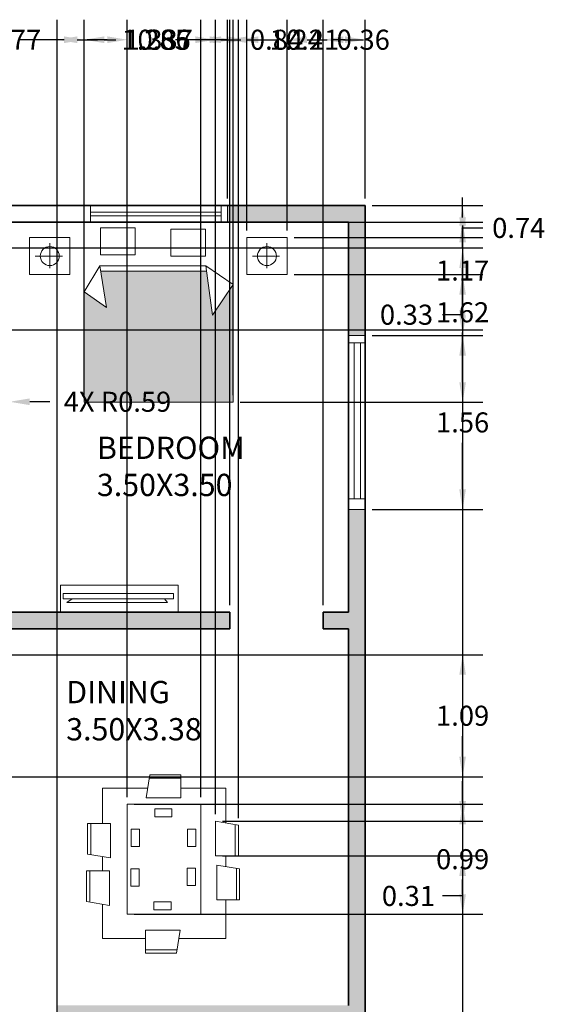
# Model space of a CAD drawing. Units: metres. Extents: x 36 to 56493, y 9 to 42849.
# Tile 5 of 5: x 56488.056 to 56492.773, y 42839.883 to 42848.722. Entities that reach past the tile are written whole.
import ezdxf

# ---------------------------------------------------------------- set-up
doc = ezdxf.new("R2010")
doc.units = ezdxf.units.M
doc.header["$MEASUREMENT"] = 0
for name, color, linetype, lineweight in [('A-ANNO-DIMS', 2, 'Continuous', 18), ('A-AREA-IDEN', 7, 'Continuous', 18), ('A-EQPM', 8, 'Continuous', 18), ('A-FURN', 8, 'Continuous', 18), ('A-FURN-PATT', 252, 'Continuous', 13), ('A-GLAZ', 4, 'Continuous', 18), ('A-WALL', 7, 'Continuous', 35)]:
    doc.layers.add(name, color=color, linetype=linetype, lineweight=lineweight)
doc.layers.add('A-WALL-PATT', color=30, linetype='Continuous', lineweight=13, true_color=0xf26722)
doc.styles.get("Standard").update_dxf_attribs({"font": 'arial.ttf'})
doc.dimstyles.get("Standard").update_dxf_attribs({"dimtxt": 0.18, "dimasz": 0.18, "dimexe": 0.18, "dimexo": 0.0625, "dimgap": 0.09, "dimtad": 0, "dimtih": 1, "dimtoh": 1, "dimdec": 0, "dimzin": 0, "dimdsep": 46, "dimtxsty": 'Standard', "dimcen": 0.09, "dimadec": 0, "dimazin": 0, "dimtfac": 1, "dimtdec": 0, "dimtofl": 0, "dimtmove": 0, "dimatfit": 3, "dimfxl": 1, "dimtolj": 1, "dimtzin": 0, "dimarcsym": 0})

# ---------------------------------------------------------------- blocks, each defined once
blk = doc.blocks.new('CHAIR-DINING')
for p, q in [((0, -0.0005), (0.0341, 0.2049)), ((0.0341, 0.2049), (0.3107, 0.2049)), ((0.3107, 0.2049), (0.3107, -0.0005)), ((0.0292, 0.1752), (0.3107, 0.1752)), ((0, -0.0005), (0.3107, -0.0005))]:
    blk.add_line(p, q)
blk = doc.blocks.new('NIGHTSTAND-COMPACT')
for p, q in [((0.1807, 0.2832), (0.1807, 0.057)), ((0.0508, 0.1663), (0.2939, 0.1663))]:
    blk.add_line(p, q)
blk.add_lwpolyline([(0, 0.3329), (0.3614, 0.3329), (0.3614, -0.0003), (0, -0.0003)], close=True)
blk.add_circle((0.1807, 0.1663), 0.0852)
blk = doc.blocks.new('*D17')
at = {"layer": 'A-ANNO-DIMS', "color": 0, "lineweight": -2, "transparency": 16777216}
for p, q in [((56491.2188, 42847.0533), (56492.2108, 42847.0533)), ((56492.0308, 42846.8733), (56492.0308, 42838.9334)), ((56492.0308, 42830.6296), (56492.0308, 42838.5695)), ((56489.3111, 42830.4496), (56492.2108, 42830.4496))]:
    blk.add_line(p, q, dxfattribs=at)
at = {"layer": 'A-ANNO-DIMS', "color": 0, "transparency": 16777216}
for points in [[(56492.0008, 42846.8733), (56492.0608, 42846.8733), (56492.0308, 42847.0533)], [(56492.0008, 42830.6296), (56492.0608, 42830.6296), (56492.0308, 42830.4496)]]:
    blk.add_solid(points, dxfattribs=at)
at = {"layer": 'Defpoints', "color": 0, "transparency": 16777216}
for p in [(56491.1563, 42847.0533), (56489.2486, 42830.4496), (56492.0308, 42830.4496)]:
    blk.add_point(p, dxfattribs=at)
at = {"layer": 'A-ANNO-DIMS', "color": 0, "transparency": 16777216, "insert": (56492.0308, 42838.7514), "char_height": 0.18, "attachment_point": 5}
blk.add_mtext('\\A1;16.604', dxfattribs=at)
blk = doc.blocks.new('*D23')
at = {"layer": 'A-ANNO-DIMS', "color": 0, "lineweight": -2, "transparency": 16777216}
for p, q in [((56489.8126, 42841.5894), (56489.8126, 42848.722)), ((56490.0179, 42841.5553), (56490.0179, 42848.722)), ((56489.6326, 42848.542), (56489.4526, 42848.542)), ((56490.1979, 42848.542), (56490.3779, 42848.542))]:
    blk.add_line(p, q, dxfattribs=at)
at = {"layer": 'A-ANNO-DIMS', "color": 0, "transparency": 16777216}
for points in [[(56489.6326, 42848.572), (56489.6326, 42848.512), (56489.8126, 42848.542)], [(56490.1979, 42848.572), (56490.1979, 42848.512), (56490.0179, 42848.542)]]:
    blk.add_solid(points, dxfattribs=at)
at = {"layer": 'Defpoints', "color": 0, "transparency": 16777216}
for p in [(56490.0179, 42848.542), (56489.8126, 42841.5269), (56490.0179, 42841.4928)]:
    blk.add_point(p, dxfattribs=at)
at = {"layer": 'A-ANNO-DIMS', "color": 0, "transparency": 16777216, "insert": (56490.6843, 42848.542), "char_height": 0.18, "attachment_point": 5}
blk.add_mtext('\\A1;0.21', dxfattribs=at)
blk = doc.blocks.new('*D24')
at = {"layer": 'A-ANNO-DIMS', "color": 0, "lineweight": -2, "transparency": 16777216}
for p, q in [((56492.0308, 42841.7069), (56492.0308, 42841.8869)), ((56489.8751, 42841.5269), (56492.2108, 42841.5269)), ((56489.8751, 42841.2162), (56492.2108, 42841.2162)), ((56492.0308, 42841.0362), (56492.0308, 42840.8562)), ((56492.0308, 42840.8562), (56491.8508, 42840.8562))]:
    blk.add_line(p, q, dxfattribs=at)
at = {"layer": 'A-ANNO-DIMS', "color": 0, "transparency": 16777216}
for points in [[(56492.0008, 42841.7069), (56492.0608, 42841.7069), (56492.0308, 42841.5269)], [(56492.0008, 42841.0362), (56492.0608, 42841.0362), (56492.0308, 42841.2162)]]:
    blk.add_solid(points, dxfattribs=at)
at = {"layer": 'Defpoints', "color": 0, "transparency": 16777216}
for p in [(56489.8126, 42841.5269), (56489.8126, 42841.2162), (56492.0308, 42841.2162)]:
    blk.add_point(p, dxfattribs=at)
at = {"layer": 'A-ANNO-DIMS', "color": 0, "transparency": 16777216, "insert": (56491.5443, 42840.8562), "char_height": 0.18, "attachment_point": 5}
blk.add_mtext('\\A1;0.31', dxfattribs=at)
blk = doc.blocks.new('*D27')
at = {"layer": 'A-ANNO-DIMS', "color": 0, "lineweight": -2, "transparency": 16777216}
for p, q in [((56490.094, 42846.8294), (56490.094, 42848.722)), ((56490.4554, 42846.8294), (56490.4554, 42848.722)), ((56489.914, 42848.542), (56489.734, 42848.542)), ((56490.6354, 42848.542), (56490.8154, 42848.542))]:
    blk.add_line(p, q, dxfattribs=at)
at = {"layer": 'A-ANNO-DIMS', "color": 0, "transparency": 16777216}
for points in [[(56489.914, 42848.572), (56489.914, 42848.512), (56490.094, 42848.542)], [(56490.6354, 42848.572), (56490.6354, 42848.512), (56490.4554, 42848.542)]]:
    blk.add_solid(points, dxfattribs=at)
at = {"layer": 'Defpoints', "color": 0, "transparency": 16777216}
for p in [(56490.4554, 42848.542), (56490.094, 42846.7669), (56490.4554, 42846.7669)]:
    blk.add_point(p, dxfattribs=at)
at = {"layer": 'A-ANNO-DIMS', "color": 0, "transparency": 16777216, "insert": (56491.1391, 42848.542), "char_height": 0.18, "attachment_point": 5}
blk.add_mtext('\\A1;0.36', dxfattribs=at)
blk = doc.blocks.new('*D28')
at = {"layer": 'A-ANNO-DIMS', "color": 0, "lineweight": -2, "transparency": 16777216}
for p, q in [((56492.030752, 42846.94694), (56492.030752, 42847.12694)), ((56490.517921, 42846.76694), (56492.210752, 42846.76694)), ((56490.517921, 42846.433723), (56492.210752, 42846.433723)), ((56492.030752, 42846.253723), (56492.030752, 42846.073723)), ((56492.030752, 42846.073723), (56491.850752, 42846.073723))]:
    blk.add_line(p, q, dxfattribs=at)
at = {"layer": 'A-ANNO-DIMS', "color": 0, "transparency": 16777216}
for points in [[(56492.000752, 42846.94694), (56492.060752, 42846.94694), (56492.030752, 42846.76694)], [(56492.000752, 42846.253723), (56492.060752, 42846.253723), (56492.030752, 42846.433723)]]:
    blk.add_solid(points, dxfattribs=at)
at = {"layer": 'Defpoints', "color": 0, "transparency": 16777216}
for p in [(56490.455421, 42846.76694), (56490.455421, 42846.433723), (56492.030752, 42846.433723)]:
    blk.add_point(p, dxfattribs=at)
at = {"layer": 'A-ANNO-DIMS', "color": 0, "transparency": 16777216, "insert": (56491.526973, 42846.073723), "char_height": 0.18, "attachment_point": 5}
blk.add_mtext('\\A1;0.33', dxfattribs=at)
blk = doc.blocks.new('*D45')
at = {"layer": 'A-ANNO-DIMS', "color": 0, "lineweight": -2, "transparency": 16777216}
for p, q in [((56486.6826, 42847.1158), (56486.6826, 42848.722)), ((56488.6347, 42847.1158), (56488.6347, 42848.722)), ((56486.8626, 42848.542), (56487.2744, 42848.542)), ((56488.4547, 42848.542), (56488.043, 42848.542))]:
    blk.add_line(p, q, dxfattribs=at)
at = {"layer": 'A-ANNO-DIMS', "color": 0, "transparency": 16777216}
for points in [[(56486.8626, 42848.572), (56486.8626, 42848.512), (56486.6826, 42848.542)], [(56488.4547, 42848.572), (56488.4547, 42848.512), (56488.6347, 42848.542)]]:
    blk.add_solid(points, dxfattribs=at)
at = {"layer": 'Defpoints', "color": 0, "transparency": 16777216}
for p in [(56488.6347, 42848.542), (56486.6826, 42847.0533), (56488.6347, 42847.0533)]:
    blk.add_point(p, dxfattribs=at)
at = {"layer": 'A-ANNO-DIMS', "color": 0, "transparency": 16777216, "insert": (56487.6587, 42848.542), "char_height": 0.18, "attachment_point": 5}
blk.add_mtext('\\A1;1.952', dxfattribs=at)
blk = doc.blocks.new('*D46')
at = {"layer": 'A-ANNO-DIMS', "color": 0, "lineweight": -2, "transparency": 16777216}
for p, q in [((56488.6347, 42847.1158), (56488.6347, 42848.722)), ((56489.9198, 42847.1158), (56489.9198, 42848.722)), ((56488.4547, 42848.542), (56488.2747, 42848.542)), ((56490.0998, 42848.542), (56490.2798, 42848.542))]:
    blk.add_line(p, q, dxfattribs=at)
at = {"layer": 'A-ANNO-DIMS', "color": 0, "transparency": 16777216}
for points in [[(56488.4547, 42848.572), (56488.4547, 42848.512), (56488.6347, 42848.542)], [(56490.0998, 42848.572), (56490.0998, 42848.512), (56489.9198, 42848.542)]]:
    blk.add_solid(points, dxfattribs=at)
at = {"layer": 'Defpoints', "color": 0, "transparency": 16777216}
for p in [(56489.9198, 42848.542), (56488.6347, 42847.0533), (56489.9198, 42847.0533)]:
    blk.add_point(p, dxfattribs=at)
at = {"layer": 'A-ANNO-DIMS', "color": 0, "transparency": 16777216, "insert": (56489.2773, 42848.542), "char_height": 0.18, "attachment_point": 5}
blk.add_mtext('\\A1;1.285', dxfattribs=at)
blk = doc.blocks.new('*D47')
at = {"layer": 'A-ANNO-DIMS', "color": 0, "lineweight": -2, "transparency": 16777216}
for p, q in [((56489.9198, 42847.1158), (56489.9198, 42848.722)), ((56491.1563, 42847.1158), (56491.1563, 42848.722)), ((56490.0998, 42848.542), (56490.2231, 42848.542)), ((56490.9763, 42848.542), (56490.853, 42848.542))]:
    blk.add_line(p, q, dxfattribs=at)
at = {"layer": 'A-ANNO-DIMS', "color": 0, "transparency": 16777216}
for points in [[(56490.0998, 42848.572), (56490.0998, 42848.512), (56489.9198, 42848.542)], [(56490.9763, 42848.572), (56490.9763, 42848.512), (56491.1563, 42848.542)]]:
    blk.add_solid(points, dxfattribs=at)
at = {"layer": 'Defpoints', "color": 0, "transparency": 16777216}
for p in [(56491.1563, 42848.542), (56489.9198, 42847.0533), (56491.1563, 42847.0533)]:
    blk.add_point(p, dxfattribs=at)
at = {"layer": 'A-ANNO-DIMS', "color": 0, "transparency": 16777216, "insert": (56490.538, 42848.542), "char_height": 0.18, "attachment_point": 5}
blk.add_mtext('\\A1;1.24', dxfattribs=at)
blk = doc.blocks.new('*D54')
at = {"layer": 'A-ANNO-DIMS', "color": 0, "lineweight": -2, "transparency": 16777216}
for p, q in [((56491.2188, 42847.0533), (56492.2108, 42847.0533)), ((56492.0308, 42846.8733), (56492.0308, 42846.6505)), ((56492.0308, 42846.067), (56492.0308, 42846.2898)), ((56491.2188, 42845.887), (56492.2108, 42845.887))]:
    blk.add_line(p, q, dxfattribs=at)
at = {"layer": 'A-ANNO-DIMS', "color": 0, "transparency": 16777216}
for points in [[(56492.0008, 42846.8733), (56492.0608, 42846.8733), (56492.0308, 42847.0533)], [(56492.0008, 42846.067), (56492.0608, 42846.067), (56492.0308, 42845.887)]]:
    blk.add_solid(points, dxfattribs=at)
at = {"layer": 'Defpoints', "color": 0, "transparency": 16777216}
for p in [(56491.1563, 42847.0533), (56491.1563, 42845.887), (56492.0308, 42845.887)]:
    blk.add_point(p, dxfattribs=at)
at = {"layer": 'A-ANNO-DIMS', "color": 0, "transparency": 16777216, "insert": (56492.0308, 42846.4701), "char_height": 0.18, "attachment_point": 5}
blk.add_mtext('\\A1;1.17', dxfattribs=at)
blk = doc.blocks.new('*D55')
at = {"layer": 'A-ANNO-DIMS', "color": 0, "lineweight": -2, "transparency": 16777216}
for p, q in [((56491.2188, 42845.887), (56492.2108, 42845.887)), ((56492.0308, 42845.707), (56492.0308, 42845.2886)), ((56492.0308, 42844.5064), (56492.0308, 42844.9248)), ((56491.2188, 42844.3264), (56492.2108, 42844.3264))]:
    blk.add_line(p, q, dxfattribs=at)
at = {"layer": 'A-ANNO-DIMS', "color": 0, "transparency": 16777216}
for points in [[(56492.0008, 42845.707), (56492.0608, 42845.707), (56492.0308, 42845.887)], [(56492.0008, 42844.5064), (56492.0608, 42844.5064), (56492.0308, 42844.3264)]]:
    blk.add_solid(points, dxfattribs=at)
at = {"layer": 'Defpoints', "color": 0, "transparency": 16777216}
for p in [(56491.1563, 42845.887), (56491.1563, 42844.3264), (56492.0308, 42844.3264)]:
    blk.add_point(p, dxfattribs=at)
at = {"layer": 'A-ANNO-DIMS', "color": 0, "transparency": 16777216, "insert": (56492.0308, 42845.1067), "char_height": 0.18, "attachment_point": 5}
blk.add_mtext('\\A1;1.56', dxfattribs=at)
blk = doc.blocks.new('*D58')
at = {"layer": 'A-ANNO-DIMS', "color": 0, "lineweight": -2, "transparency": 16777216}
for p, q in [((56488.6347, 42845.3504), (56488.6347, 42848.722)), ((56489.9717, 42845.3504), (56489.9717, 42848.722)), ((56488.8147, 42848.542), (56488.918, 42848.542)), ((56489.7917, 42848.542), (56489.6885, 42848.542))]:
    blk.add_line(p, q, dxfattribs=at)
at = {"layer": 'A-ANNO-DIMS', "color": 0, "transparency": 16777216}
for points in [[(56488.8147, 42848.572), (56488.8147, 42848.512), (56488.6347, 42848.542)], [(56489.7917, 42848.572), (56489.7917, 42848.512), (56489.9717, 42848.542)]]:
    blk.add_solid(points, dxfattribs=at)
at = {"layer": 'Defpoints', "color": 0, "transparency": 16777216}
for p in [(56489.9717, 42848.542), (56488.6347, 42845.2879), (56489.9717, 42845.2879)]:
    blk.add_point(p, dxfattribs=at)
at = {"layer": 'A-ANNO-DIMS', "color": 0, "transparency": 16777216, "insert": (56489.3032, 42848.542), "char_height": 0.18, "attachment_point": 5}
blk.add_mtext('\\A1;1.337', dxfattribs=at)
blk = doc.blocks.new('*D59')
at = {"layer": 'A-ANNO-DIMS', "color": 0, "lineweight": -2, "transparency": 16777216}
for p, q in [((56490.0342, 42846.9033), (56492.2108, 42846.9033)), ((56492.0308, 42846.7233), (56492.0308, 42846.2775)), ((56492.0308, 42845.4679), (56492.0308, 42845.9137)), ((56490.0342, 42845.2879), (56492.2108, 42845.2879))]:
    blk.add_line(p, q, dxfattribs=at)
at = {"layer": 'A-ANNO-DIMS', "color": 0, "transparency": 16777216}
for points in [[(56492.0008, 42846.7233), (56492.0608, 42846.7233), (56492.0308, 42846.9033)], [(56492.0008, 42845.4679), (56492.0608, 42845.4679), (56492.0308, 42845.2879)]]:
    blk.add_solid(points, dxfattribs=at)
at = {"layer": 'Defpoints', "color": 0, "transparency": 16777216}
for p in [(56489.9717, 42846.9033), (56492.0308, 42846.9033), (56489.9717, 42845.2879)]:
    blk.add_point(p, dxfattribs=at)
at = {"layer": 'A-ANNO-DIMS', "color": 0, "transparency": 16777216, "insert": (56492.0308, 42846.0956), "char_height": 0.18, "attachment_point": 5}
blk.add_mtext('\\A1;1.62', dxfattribs=at)
blk = doc.blocks.new('*D60')
at = {"layer": 'A-ANNO-DIMS', "color": 0, "lineweight": -2, "transparency": 16777216}
for p, q in [((56489.021472, 42841.742527), (56489.021472, 42848.721953)), ((56489.681318, 42841.742527), (56489.681318, 42848.721953)), ((56488.841472, 42848.541953), (56488.661472, 42848.541953)), ((56489.861318, 42848.541953), (56490.041318, 42848.541953))]:
    blk.add_line(p, q, dxfattribs=at)
at = {"layer": 'A-ANNO-DIMS', "color": 0, "transparency": 16777216}
for points in [[(56488.841472, 42848.571953), (56488.841472, 42848.511953), (56489.021472, 42848.541953)], [(56489.861318, 42848.571953), (56489.861318, 42848.511953), (56489.681318, 42848.541953)]]:
    blk.add_solid(points, dxfattribs=at)
at = {"layer": 'Defpoints', "color": 0, "transparency": 16777216}
for p in [(56489.681318, 42848.541953), (56489.021472, 42841.680027), (56489.681318, 42841.680027)]:
    blk.add_point(p, dxfattribs=at)
at = {"layer": 'A-ANNO-DIMS', "color": 0, "transparency": 16777216, "insert": (56489.351395, 42848.541953), "char_height": 0.18, "attachment_point": 5}
blk.add_mtext('\\A1;0.66', dxfattribs=at)
blk = doc.blocks.new('*D61')
at = {"layer": 'A-ANNO-DIMS', "color": 0, "lineweight": -2, "transparency": 16777216}
for p, q in [((56489.084, 42841.68), (56492.2108, 42841.68)), ((56492.0308, 42841.5), (56492.0308, 42841.3677)), ((56492.0308, 42840.8715), (56492.0308, 42841.0039)), ((56489.084, 42840.6915), (56492.2108, 42840.6915))]:
    blk.add_line(p, q, dxfattribs=at)
at = {"layer": 'A-ANNO-DIMS', "color": 0, "transparency": 16777216}
for points in [[(56492.0008, 42841.5), (56492.0608, 42841.5), (56492.0308, 42841.68)], [(56492.0008, 42840.8715), (56492.0608, 42840.8715), (56492.0308, 42840.6915)]]:
    blk.add_solid(points, dxfattribs=at)
at = {"layer": 'Defpoints', "color": 0, "transparency": 16777216}
for p in [(56489.0215, 42841.68), (56489.0215, 42840.6915), (56492.0308, 42840.6915)]:
    blk.add_point(p, dxfattribs=at)
at = {"layer": 'A-ANNO-DIMS', "color": 0, "transparency": 16777216, "insert": (56492.0308, 42841.1858), "char_height": 0.18, "attachment_point": 5}
blk.add_mtext('\\A1;0.99', dxfattribs=at)
blk = doc.blocks.new('*D63')
at = {"layer": 'A-ANNO-DIMS', "color": 0, "lineweight": -2, "transparency": 16777216}
for p, q in [((56492.0308, 42846.6728), (56492.0308, 42846.8528)), ((56492.0308, 42846.8528), (56492.2108, 42846.8528)), ((56487.4188, 42846.6728), (56492.2108, 42846.6728)), ((56492.0308, 42846.1166), (56492.0308, 42846.4928)), ((56487.4188, 42845.9366), (56492.2108, 42845.9366))]:
    blk.add_line(p, q, dxfattribs=at)
at = {"layer": 'A-ANNO-DIMS', "color": 0, "transparency": 16777216}
for points in [[(56492.0008, 42846.4928), (56492.0608, 42846.4928), (56492.0308, 42846.6728)], [(56492.0008, 42846.1166), (56492.0608, 42846.1166), (56492.0308, 42845.9366)]]:
    blk.add_solid(points, dxfattribs=at)
at = {"layer": 'Defpoints', "color": 0, "transparency": 16777216}
for p in [(56487.3563, 42846.6728), (56492.0308, 42846.6728), (56487.3563, 42845.9366)]:
    blk.add_point(p, dxfattribs=at)
at = {"layer": 'A-ANNO-DIMS', "color": 0, "transparency": 16777216, "insert": (56492.5342, 42846.8528), "char_height": 0.18, "attachment_point": 5}
blk.add_mtext('\\A1;0.74', dxfattribs=at)
blk = doc.blocks.new('*D64')
at = {"layer": 'A-ANNO-DIMS', "color": 0, "lineweight": -2, "transparency": 16777216}
for p, q in [((56487.4188, 42843.021), (56492.2108, 42843.021)), ((56492.0308, 42842.841), (56492.0308, 42842.6556)), ((56492.0308, 42842.1064), (56492.0308, 42842.2918)), ((56487.4188, 42841.9264), (56492.2108, 42841.9264))]:
    blk.add_line(p, q, dxfattribs=at)
at = {"layer": 'A-ANNO-DIMS', "color": 0, "transparency": 16777216}
for points in [[(56492.0008, 42842.841), (56492.0608, 42842.841), (56492.0308, 42843.021)], [(56492.0008, 42842.1064), (56492.0608, 42842.1064), (56492.0308, 42841.9264)]]:
    blk.add_solid(points, dxfattribs=at)
at = {"layer": 'Defpoints', "color": 0, "transparency": 16777216}
for p in [(56487.3563, 42843.021), (56487.3563, 42841.9264), (56492.0308, 42841.9264)]:
    blk.add_point(p, dxfattribs=at)
at = {"layer": 'A-ANNO-DIMS', "color": 0, "transparency": 16777216, "insert": (56492.0308, 42842.4737), "char_height": 0.18, "attachment_point": 5}
blk.add_mtext('\\A1;1.09', dxfattribs=at)
blk = doc.blocks.new('*D65')
at = {"layer": 'A-ANNO-DIMS', "color": 0, "lineweight": -2, "transparency": 16777216}
for p, q in [((56489.940126, 42843.465791), (56489.940126, 42848.721953)), ((56490.780472, 42843.465791), (56490.780472, 42848.721953)), ((56489.760126, 42848.541953), (56489.580126, 42848.541953)), ((56490.960472, 42848.541953), (56491.140472, 42848.541953))]:
    blk.add_line(p, q, dxfattribs=at)
at = {"layer": 'A-ANNO-DIMS', "color": 0, "transparency": 16777216}
for points in [[(56489.760126, 42848.571953), (56489.760126, 42848.511953), (56489.940126, 42848.541953)], [(56490.960472, 42848.571953), (56490.960472, 42848.511953), (56490.780472, 42848.541953)]]:
    blk.add_solid(points, dxfattribs=at)
at = {"layer": 'Defpoints', "color": 0, "transparency": 16777216}
for p in [(56490.780472, 42848.541953), (56489.940126, 42843.403291), (56490.780472, 42843.403291)]:
    blk.add_point(p, dxfattribs=at)
at = {"layer": 'A-ANNO-DIMS', "color": 0, "transparency": 16777216, "insert": (56490.360299, 42848.541953), "char_height": 0.18, "attachment_point": 5}
blk.add_mtext('\\A1;0.84', dxfattribs=at)
blk = doc.blocks.new('*D67')
at = {"layer": 'A-ANNO-DIMS', "color": 0, "lineweight": -2, "transparency": 16777216}
for p, q in [((56487.626252, 42839.785791), (56487.626252, 42848.721953)), ((56488.392626, 42839.785791), (56488.392626, 42848.721953)), ((56487.446252, 42848.541953), (56487.266252, 42848.541953)), ((56488.572626, 42848.541953), (56488.752626, 42848.541953))]:
    blk.add_line(p, q, dxfattribs=at)
at = {"layer": 'A-ANNO-DIMS', "color": 0, "transparency": 16777216}
for points in [[(56487.446252, 42848.571953), (56487.446252, 42848.511953), (56487.626252, 42848.541953)], [(56488.572626, 42848.571953), (56488.572626, 42848.511953), (56488.392626, 42848.541953)]]:
    blk.add_solid(points, dxfattribs=at)
at = {"layer": 'Defpoints', "color": 0, "transparency": 16777216}
for p in [(56488.392626, 42848.541953), (56487.626252, 42839.723291), (56488.392626, 42839.723291)]:
    blk.add_point(p, dxfattribs=at)
at = {"layer": 'A-ANNO-DIMS', "color": 0, "transparency": 16777216, "insert": (56488.009439, 42848.541953), "char_height": 0.18, "attachment_point": 5}
blk.add_mtext('\\A1;0.77', dxfattribs=at)
blk = doc.blocks.new('*D71')
at = {"layer": 'A-ANNO-DIMS', "color": 0, "lineweight": -2, "transparency": 16777216}
for p, q in [((56487.3732, 42845.2016), (56487.3732, 42845.3816)), ((56487.2832, 42845.2916), (56487.4632, 42845.2916)), ((56488.3266, 42845.2922), (56488.1466, 42845.2921))]:
    blk.add_line(p, q, dxfattribs=at)
at = {"layer": 'A-ANNO-DIMS', "color": 0, "transparency": 16777216}
blk.add_solid([(56488.1466, 42845.3221), (56488.1466, 42845.2621), (56487.9666, 42845.292)], dxfattribs=at)
at = {"layer": 'Defpoints', "color": 0, "transparency": 16777216}
for p in [(56487.3732, 42845.2916), (56487.9666, 42845.292)]:
    blk.add_point(p, dxfattribs=at)
at = {"layer": 'A-ANNO-DIMS', "color": 0, "transparency": 16777216, "insert": (56488.9337, 42845.2922), "char_height": 0.18, "attachment_point": 5}
blk.add_mtext('\\A1;4X R0.59', dxfattribs=at)

msp = doc.modelspace()

# ---------------------------------------------------------------- hatches: boundary and pattern name
at = {"layer": 'A-FURN-PATT'}
h = msp.add_hatch(color=256, dxfattribs=at)
h.dxf.hatch_style = 1
h.paths.add_polyline_path([(56489.9717, 42846.3436), (56489.785, 42846.0689), (56489.7313, 42846.464), (56488.7831, 42846.4638), (56488.8356, 42846.1393), (56488.6347, 42846.2795), (56488.6347, 42845.2879), (56489.9717, 42845.2879)])
at = {"layer": 'A-WALL-PATT'}
h = msp.add_hatch(color=256, dxfattribs=at)
h.dxf.hatch_style = 1
edge = h.paths.add_edge_path()
edge.add_line((56483.5429, 42845.6533), (56483.4063, 42845.6533))
edge.add_line((56483.4063, 42845.6533), (56483.4063, 42846.9033))
edge.add_line((56483.4063, 42846.9033), (56483.63, 42846.9033))
edge.add_ellipse((56483.6664, 42846.7323), major_axis=(0.2141, -0.003), ratio=0.809245, start_angle=94.07135, end_angle=102.818, ccw=False)
edge.add_line((56483.6565, 42846.9062), (56483.6565, 42846.9056))
edge.add_line((56483.6565, 42846.9056), (56483.6615, 42846.9056))
edge.add_ellipse((56483.6664, 42846.7323), major_axis=(0.2141, -0.003), ratio=0.809245, start_angle=90, end_angle=92.42655, ccw=False)
edge.add_line((56483.6812, 42846.9058), (56483.6812, 42846.9052))
edge.add_ellipse((56483.6664, 42846.7323), major_axis=(0.2141, -0.003), ratio=0.809245, start_angle=79.57494, end_angle=85.92601, ccw=False)
edge.add_line((56483.7048, 42846.9033), (56484.1418, 42846.9033))
edge.add_line((56484.1418, 42846.9033), (56484.1418, 42847.0533))
edge.add_line((56484.1418, 42847.0533), (56483.2563, 42847.0533))
edge.add_line((56483.2563, 42847.0533), (56483.2563, 42844.1391))
edge.add_line((56483.2563, 42844.1391), (56483.4063, 42844.1391))
edge.add_line((56483.4063, 42844.1391), (56483.4063, 42844.2368))
edge.add_line((56483.4063, 42844.2368), (56483.4063, 42845.5033))
edge.add_line((56483.4063, 42845.5033), (56483.5429, 42845.5033))
edge.add_line((56483.5429, 42845.5033), (56483.5429, 42845.6533))
edge = h.paths.add_edge_path(flags=0)
edge.add_line((56488.6347, 42847.0533), (56486.6826, 42847.0533))
edge.add_line((56486.6826, 42847.0533), (56486.6826, 42846.9033))
edge.add_line((56486.6826, 42846.9033), (56486.9892, 42846.9033))
edge.add_ellipse((56487.0257, 42846.7323), major_axis=(0.2141, -0.003), ratio=0.809245, start_angle=94.07135, end_angle=102.818, ccw=False)
edge.add_line((56487.0157, 42846.9062), (56487.0157, 42846.9056))
edge.add_line((56487.0157, 42846.9056), (56487.0207, 42846.9056))
edge.add_ellipse((56487.0257, 42846.7323), major_axis=(0.2141, -0.003), ratio=0.809245, start_angle=90, end_angle=92.42655, ccw=False)
edge.add_line((56487.0404, 42846.9058), (56487.0404, 42846.9052))
edge.add_ellipse((56487.0257, 42846.7323), major_axis=(0.2141, -0.003), ratio=0.809245, start_angle=79.57494, end_angle=85.92601, ccw=False)
edge.add_line((56487.064, 42846.9033), (56487.3563, 42846.9033))
edge.add_line((56487.3563, 42846.9033), (56487.3563, 42846.6728))
edge.add_line((56487.3563, 42846.6728), (56487.5063, 42846.6728))
edge.add_line((56487.5063, 42846.6728), (56487.5063, 42846.9033))
edge.add_line((56487.5063, 42846.9033), (56488.6347, 42846.9033))
edge.add_line((56488.6347, 42846.9033), (56488.6347, 42847.0533))
h.paths.add_polyline_path([(56486.2245, 42847.0533), (56484.665, 42847.0533), (56484.665, 42846.9033), (56485.4063, 42846.9033), (56485.4063, 42845.6533), (56484.2087, 42845.6533), (56484.2087, 42845.5033), (56487.3563, 42845.5033), (56487.3563, 42844.954), (56487.3563, 42843.021), (56487.5063, 42843.021), (56487.5063, 42843.2533), (56489.9401, 42843.2533), (56489.9401, 42843.4033), (56487.5063, 42843.4033), (56487.5063, 42845.6238), (56487.5063, 42845.6533), (56487.5063, 42845.9366), (56487.3563, 42845.9366), (56487.3563, 42845.6533), (56485.5563, 42845.6533), (56485.5563, 42846.9033), (56486.2245, 42846.9033)])
h.paths.add_polyline_path([(56491.1563, 42847.0533), (56489.9198, 42847.0533), (56489.9198, 42846.9033), (56489.9717, 42846.9033), (56491.0063, 42846.9033), (56491.0063, 42845.887), (56491.1563, 42845.887)])
h.paths.add_polyline_path([(56491.1563, 42844.3264), (56491.0063, 42844.3264), (56491.0063, 42843.4033), (56490.7805, 42843.4033), (56490.7805, 42843.2533), (56491.0063, 42843.2533), (56491.0063, 42839.8733), (56488.3926, 42839.8733), (56488.3926, 42839.7233), (56491.0063, 42839.7233), (56491.0063, 42836.1233), (56487.6263, 42836.1233), (56487.6263, 42839.0009), (56487.4763, 42839.0009), (56487.4763, 42836.1233), (56486.4863, 42836.1233), (56486.4863, 42835.9733), (56487.4763, 42835.9733), (56487.8849, 42835.9733), (56487.8849, 42832.9233), (56487.8913, 42832.9233), (56488.0349, 42832.9233), (56488.0349, 42833.0733), (56488.0349, 42835.9733), (56491.0063, 42835.9733), (56491.0063, 42833.0733), (56491.0063, 42832.9233), (56491.1563, 42832.9233), (56491.1563, 42835.9733)])
h.paths.add_polyline_path([(56483.4063, 42842.8378), (56483.2563, 42842.8378), (56483.2563, 42841.5433), (56483.2563, 42840.8898), (56483.4063, 42840.8898), (56483.4063, 42841.3933), (56485.0063, 42841.3933), (56485.0063, 42841.2426), (56485.1563, 42841.2426), (56485.1563, 42841.3933), (56487.3563, 42841.3933), (56487.5063, 42841.3933), (56487.5063, 42841.9264), (56487.3563, 42841.9264), (56487.3563, 42841.5433), (56483.4063, 42841.5433)])
h.paths.add_polyline_path([(56485.1563, 42840.351), (56485.0063, 42840.351), (56485.0063, 42839.8933), (56483.4063, 42839.8933), (56483.4063, 42840.3779), (56483.2563, 42840.3779), (56483.2563, 42839.8933), (56483.2563, 42838.6997), (56483.4063, 42838.6997), (56483.4063, 42839.7433), (56485.1563, 42839.7433)])
h.paths.add_polyline_path([(56483.4063, 42836.7612), (56483.2563, 42836.7612), (56483.2563, 42835.6733), (56483.2563, 42834.2533), (56483.2563, 42832.9233), (56485.9871, 42832.9233), (56485.9871, 42833.0733), (56483.4063, 42833.0733), (56483.4063, 42834.2533), (56483.4063, 42835.5233), (56485.4763, 42835.5233), (56485.9871, 42835.5233), (56485.9871, 42835.6733), (56485.6263, 42835.6733), (56483.4063, 42835.6733)])

# ---------------------------------------------------------------- linework, layer by layer
at = {"layer": 'A-EQPM'}
for p, q in [((56488.5276, 42843.5246), (56488.4796, 42843.4911)), ((56488.4796, 42843.4911), (56489.3827, 42843.4911)), ((56489.3827, 42843.4911), (56489.3543, 42843.5246))]:
    msp.add_line(p, q, dxfattribs=at)
for points in [[(56488.4205, 42843.4033), (56489.4788, 42843.4033), (56489.4788, 42843.6458), (56488.4205, 42843.6458)], [(56488.4465, 42843.5711), (56489.4359, 42843.5711), (56489.4359, 42843.5246), (56488.4465, 42843.5246)]]:
    msp.add_lwpolyline(points, close=True, dxfattribs=at)
at = {"layer": 'A-FURN'}
for p, q in [((56488.7754, 42846.5115), (56488.6347, 42846.2795)), ((56488.7754, 42846.5115), (56489.7249, 42846.5115)), ((56488.8356, 42846.1393), (56488.7754, 42846.5115)), ((56489.7249, 42846.5115), (56489.9717, 42846.3436)), ((56489.785, 42846.0689), (56489.7249, 42846.5115)), ((56488.7831, 42846.4638), (56489.7313, 42846.464)), ((56489.9717, 42846.3436), (56489.785, 42846.0689)), ((56488.6347, 42846.2795), (56488.8356, 42846.1393))]:
    msp.add_line(p, q, dxfattribs=at)
for points in [[(56488.6347, 42846.9033), (56489.9717, 42846.9033), (56489.9717, 42845.2879), (56488.6347, 42845.2879)], [(56488.7796, 42846.8538), (56489.0914, 42846.8538), (56489.0914, 42846.6116), (56488.7796, 42846.6116)], [(56489.4128, 42846.8407), (56489.7246, 42846.8407), (56489.7246, 42846.5985), (56489.4128, 42846.5985)], [(56489.0215, 42841.68), (56489.6813, 42841.68), (56489.6813, 42840.6915), (56489.0215, 42840.6915)], [(56489.2673, 42841.6387), (56489.4225, 42841.6387), (56489.4225, 42841.5648), (56489.2673, 42841.5648)], [(56489.1311, 42841.454), (56489.1311, 42841.2988), (56489.0573, 42841.2988), (56489.0573, 42841.454)], [(56489.6363, 42841.4564), (56489.6363, 42841.3011), (56489.5624, 42841.3011), (56489.5624, 42841.4564)], [(56489.1264, 42841.098), (56489.1264, 42840.9427), (56489.0525, 42840.9427), (56489.0525, 42841.098)], [(56489.6339, 42841.1051), (56489.6339, 42840.9498), (56489.5601, 42840.9498), (56489.5601, 42841.1051)], [(56489.2608, 42840.8042), (56489.4161, 42840.8042), (56489.4161, 42840.7304), (56489.2608, 42840.7304)]]:
    msp.add_lwpolyline(points, close=True, dxfattribs=at)
for points in [[(56488.7998, 42841.5077), (56488.7998, 42841.8244), (56489.2054, 42841.8244)], [(56489.5017, 42841.8244), (56489.9055, 42841.8244), (56489.9055, 42841.5114)], [(56488.7998, 42841.0822), (56488.7998, 42841.2087)], [(56489.9055, 42841.2162), (56489.9055, 42841.1186)], [(56489.9055, 42840.8214), (56489.9055, 42840.4726), (56489.4836, 42840.4726)], [(56489.1855, 42840.4726), (56488.7998, 42840.4726), (56488.7998, 42840.7818)]]:
    msp.add_lwpolyline(points, dxfattribs=at)
at = {"layer": 'A-GLAZ'}
for p, q in [((56488.6347, 42847.0533), (56488.6347, 42846.9033)), ((56488.6908, 42847.0533), (56488.6908, 42846.9033)), ((56489.8629, 42847.0533), (56489.8629, 42846.9033)), ((56489.9198, 42847.0533), (56489.9198, 42846.9033)), ((56488.6908, 42846.994), (56489.8629, 42846.994)), ((56488.6908, 42846.961), (56489.8629, 42846.961)), ((56491.0063, 42845.887), (56491.1563, 42845.887)), ((56491.0063, 42845.8203), (56491.1563, 42845.8203)), ((56491.0565, 42845.8203), (56491.0565, 42844.4215)), ((56491.1143, 42845.8203), (56491.1143, 42844.4215)), ((56491.0063, 42844.4215), (56491.1563, 42844.4215)), ((56491.0063, 42844.3264), (56491.1563, 42844.3264))]:
    msp.add_line(p, q, dxfattribs=at)
at = {"layer": 'A-WALL'}
for p, q in [((56483.2563, 42847.0533), (56491.1563, 42847.0533)), ((56491.1563, 42847.0533), (56491.1563, 42843.4033)), ((56491.1563, 42847.0533), (56491.1563, 42832.9233)), ((56487.5063, 42846.9033), (56491.0063, 42846.9033)), ((56491.0063, 42846.9033), (56491.0063, 42843.4033)), ((56489.9401, 42843.4033), (56487.5063, 42843.4033)), ((56489.9401, 42843.4033), (56489.9401, 42843.2533)), ((56491.0063, 42843.4033), (56490.7805, 42843.4033)), ((56490.7805, 42843.4033), (56490.7805, 42843.2533)), ((56489.9401, 42843.2533), (56487.5063, 42843.2533)), ((56491.0063, 42843.2533), (56490.7805, 42843.2533)), ((56491.0063, 42843.2533), (56491.0063, 42839.8733))]:
    msp.add_line(p, q, dxfattribs=at)

# ---------------------------------------------------------------- block references
at = {"layer": 'A-FURN'}
for name, p in [('NIGHTSTAND-COMPACT', (56488.1449, 42846.434)), ('NIGHTSTAND-COMPACT', (56490.094, 42846.434)), ('CHAIR-DINING', (56489.191, 42841.738))]:
    msp.add_blockref(name, p, dxfattribs=at)
for p, rotation in [((56489.8131, 42841.5269), 270.0000000102918), ((56488.8696, 42841.197), 90), ((56489.8249, 42841.1321), 270.0000000057421), ((56488.861, 42840.7716), 90.0000000004862), ((56489.4962, 42840.5478), 180)]:
    msp.add_blockref('CHAIR-DINING', p, dxfattribs=dict(at, rotation=rotation))

# ---------------------------------------------------------------- texts
at = {"layer": 'A-AREA-IDEN', "char_height": 0.2, "attachment_point": 1}
for s, insert in [('BEDROOM\\P3.50X3.50', (56488.7487, 42844.9789)), ('DINING\\P3.50X3.38', (56488.473, 42842.786))]:
    msp.add_mtext_dynamic_manual_height_columns(s, width=0.817901, gutter_width=1, heights=[0], dxfattribs=dict(at, insert=insert))

# ---------------------------------------------------------------- dimensions: what is measured, and where the dimension line sits
at = {"layer": 'A-ANNO-DIMS'}
for base, p1, p2, override, picture, middle in [((56488.6347, 42848.542), (56486.6826, 42847.0533), (56488.6347, 42847.0533), {"dimdec": 3, "dimlfac": 1, "dimrnd": 0, "dimzin": 0, "dimdsep": 46, "dimlunit": 2}, '*D45', (56487.6587, 42848.542)), ((56488.3926, 42848.542), (56487.6263, 42839.7233), (56488.3926, 42839.7233), {"dimdec": 2, "dimlfac": 1, "dimrnd": 0, "dimzin": 0, "dimdsep": 46, "dimlunit": 2}, '*D67', (56488.0094, 42848.542)), ((56489.9198, 42848.542), (56488.6347, 42847.0533), (56489.9198, 42847.0533), {"dimdec": 3, "dimlfac": 1, "dimrnd": 0, "dimzin": 0, "dimdsep": 46, "dimlunit": 2}, '*D46', (56489.2773, 42848.542)), ((56489.9717, 42848.542), (56488.6347, 42845.2879), (56489.9717, 42845.2879), {"dimdec": 3, "dimlfac": 1, "dimrnd": 0, "dimzin": 0, "dimdsep": 46, "dimlunit": 2}, '*D58', (56489.3032, 42848.542)), ((56489.6813, 42848.542), (56489.0215, 42841.68), (56489.6813, 42841.68), {"dimdec": 2, "dimlfac": 1, "dimrnd": 0, "dimzin": 0, "dimdsep": 46, "dimlunit": 2}, '*D60', (56489.3514, 42848.542)), ((56490.0179, 42848.542), (56489.8126, 42841.5269), (56490.0179, 42841.4928), {"dimdec": 2, "dimlfac": 1, "dimrnd": 0, "dimzin": 0, "dimdsep": 46, "dimlunit": 2}, '*D23', (56490.6843, 42848.542)), ((56490.7805, 42848.542), (56489.9401, 42843.4033), (56490.7805, 42843.4033), {"dimdec": 2, "dimlfac": 1, "dimrnd": 0, "dimzin": 0, "dimdsep": 46, "dimlunit": 2}, '*D65', (56490.3603, 42848.542)), ((56490.4554, 42848.542), (56490.094, 42846.7669), (56490.4554, 42846.7669), {"dimdec": 2, "dimlfac": 1, "dimrnd": 0, "dimzin": 0, "dimdsep": 46, "dimlunit": 2}, '*D27', (56491.1391, 42848.542)), ((56491.1563, 42848.542), (56489.9198, 42847.0533), (56491.1563, 42847.0533), {"dimdec": 2, "dimlfac": 1, "dimrnd": 0, "dimzin": 0, "dimdsep": 46, "dimlunit": 2}, '*D47', (56490.538, 42848.542))]:
    dim = msp.add_linear_dim(base=base, p1=p1, p2=p2, dimstyle='Standard', override=override, dxfattribs=at)
    dim.commit()
    dim.dimension.update_dxf_attribs({"geometry": picture, "text_midpoint": middle})
for base, p1, p2, override, picture, middle in [((56492.0308, 42846.4337), (56490.4554, 42846.7669), (56490.4554, 42846.4337), {"dimdec": 2, "dimlfac": 1, "dimrnd": 0, "dimzin": 0, "dimdsep": 46, "dimlunit": 2}, '*D28', (56491.527, 42846.0737)), ((56492.0308, 42830.4496), (56491.1563, 42847.0533), (56489.2486, 42830.4496), {"dimdec": 3, "dimlfac": 1, "dimrnd": 0, "dimzin": 0, "dimdsep": 46, "dimlunit": 2}, '*D17', (56492.0308, 42838.7514)), ((56492.0308, 42845.887), (56491.1563, 42847.0533), (56491.1563, 42845.887), {"dimdec": 2, "dimlfac": 1, "dimrnd": 0, "dimzin": 0, "dimdsep": 46, "dimlunit": 2}, '*D54', (56492.0308, 42846.4701)), ((56492.0308, 42846.6728), (56487.3563, 42845.9366), (56487.3563, 42846.6728), {"dimdec": 2, "dimlfac": 1, "dimrnd": 0, "dimzin": 0, "dimdsep": 46, "dimlunit": 2}, '*D63', (56492.5342, 42846.8528)), ((56492.0308, 42846.9033), (56489.9717, 42845.2879), (56489.9717, 42846.9033), {"dimdec": 2, "dimlfac": 1, "dimrnd": 0, "dimzin": 0, "dimdsep": 46, "dimlunit": 2}, '*D59', (56492.0308, 42846.0956)), ((56492.0308, 42844.3264), (56491.1563, 42845.887), (56491.1563, 42844.3264), {"dimdec": 2, "dimlfac": 1, "dimrnd": 0, "dimzin": 0, "dimdsep": 46, "dimlunit": 2}, '*D55', (56492.0308, 42845.1067)), ((56492.0308, 42841.9264), (56487.3563, 42843.021), (56487.3563, 42841.9264), {"dimdec": 2, "dimlfac": 1, "dimrnd": 0, "dimzin": 0, "dimdsep": 46, "dimlunit": 2}, '*D64', (56492.0308, 42842.4737)), ((56492.0308, 42841.2162), (56489.8126, 42841.5269), (56489.8126, 42841.2162), {"dimdec": 2, "dimlfac": 1, "dimrnd": 0, "dimzin": 0, "dimdsep": 46, "dimlunit": 2}, '*D24', (56491.5443, 42840.8562)), ((56492.0308, 42840.6915), (56489.0215, 42841.68), (56489.0215, 42840.6915), {"dimdec": 2, "dimlfac": 1, "dimrnd": 0, "dimzin": 0, "dimdsep": 46, "dimlunit": 2}, '*D61', (56492.0308, 42841.1858))]:
    dim = msp.add_linear_dim(base=base, p1=p1, p2=p2, angle=90, dimstyle='Standard', override=override, dxfattribs=at)
    dim.commit()
    dim.dimension.update_dxf_attribs({"geometry": picture, "text_midpoint": middle})
dim = msp.add_radius_dim(center=(56487.3732, 42845.2916), mpoint=(56487.9666, 42845.292), text='4X <>', dimstyle='Standard', override={"dimdec": 2, "dimlfac": 1, "dimrnd": 0, "dimzin": 0, "dimdsep": 46, "dimlunit": 2}, dxfattribs=at)
dim.commit()
dim.dimension.update_dxf_attribs({"geometry": '*D71', "text_midpoint": (56488.9337, 42845.2922)})

doc.saveas('drawing.dxf')
